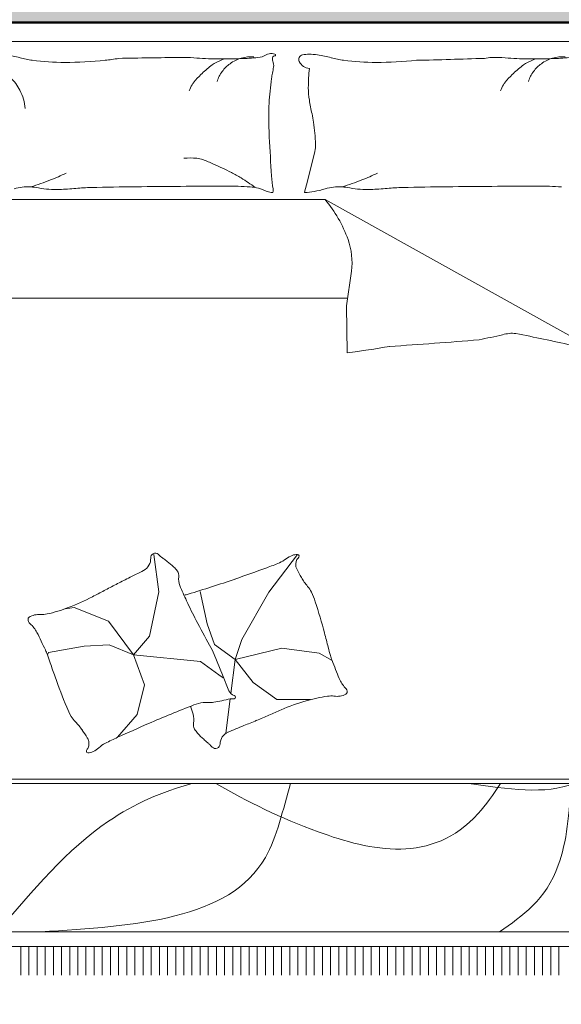
# Model space of a CAD drawing. Units: inches. Extents: x -7 to 1228, y -146 to 1091.
# Tile 11 of 88: x 105 to 153, y 401 to 487. Entities that reach past the tile are written whole.
import ezdxf

# ---------------------------------------------------------------- set-up
doc = ezdxf.new("R2010")
doc.units = ezdxf.units.IN
for name, color, linetype, lineweight in [('A-ANNO-DIMS', 2, 'Continuous', 18), ('A-FURN', 8, 'Continuous', 18), ('A-WALL', 7, 'Continuous', 50), ('A-WALL-PATT', 251, 'Continuous', 13)]:
    doc.layers.add(name, color=color, linetype=linetype, lineweight=lineweight)
doc.styles.add('DIM_FONT', font='SIMPLEX.shx', dxfattribs={"width": 0.8})
doc.styles.get("Standard").update_dxf_attribs({"font": 'arial.ttf'})
doc.dimstyles.new('ISO-25', dxfattribs={"dimtxt": 7, "dimasz": 4, "dimexe": 1.25, "dimexo": 0.625, "dimtad": 1, "dimdec": 1, "dimlunit": 3, "dimtxsty": 'Standard', "dimcen": 2.5, "dimadec": 0, "dimazin": 0, "dimtfac": 1, "dimtdec": 1, "dimtmove": 1, "dimatfit": 3, "dimfxl": 1, "dimarcsym": 0})

# ---------------------------------------------------------------- blocks, each defined once
blk = doc.blocks.new('A$C4F634EDD')
for p, q in [((0.5, 2.6295), (2.3, 2.6295)), ((0.5, 2.5771), (2.3, 2.5771)), ((1.4546, 2.1912), (1.4752, 2.2738)), ((1.4471, 2.1612), (1.4546, 2.1912)), ((1.5035, 2.141), (0.5458, 2.141)), ((1.5035, 2.141), (2.2716, 1.7136)), ((1.576, 1.9433), (1.5624, 1.8479)), ((0.5458, 1.8684), (1.5653, 1.8684)), ((1.5624, 1.8479), (1.5641, 1.7178)), ((1.031, 1.1612), (1.0448, 1.0581)), ((1.4276, 1.1611), (1.3484, 1.0571)), ((1.0448, 1.0581), (1.019, 0.936)), ((1.1784, 0.9702), (1.1586, 1.0591)), ((1.3484, 1.0571), (1.2733, 0.9268)), ((0.8108, 1.0151), (0.7868, 1.0117)), ((0.9054, 0.9773), (0.8108, 1.0151)), ((0.9743, 0.8845), (0.9054, 0.9773)), ((1.1982, 0.9129), (1.1784, 0.9702)), ((1.019, 0.936), (0.9743, 0.8845)), ((1.2733, 0.9268), (1.2555, 0.8715)), ((0.8384, 0.9085), (0.7403, 0.8913)), ((0.9072, 0.912), (0.8384, 0.9085)), ((0.9743, 0.8845), (0.9072, 0.912)), ((1.2555, 0.8715), (1.1982, 0.9129)), ((1.2555, 0.8715), (1.384, 0.9031)), ((1.384, 0.9031), (1.4868, 0.8892)), ((0.7403, 0.8913), (0.737, 0.8849)), ((0.9743, 0.8845), (1.0052, 0.802)), ((0.9743, 0.8845), (1.16, 0.8656)), ((1.1973, 0.8853), (1.2203, 0.829)), ((1.2555, 0.8715), (1.2437, 0.7773)), ((1.2555, 0.8715), (1.3049, 0.8082)), ((1.4868, 0.8892), (1.5228, 0.8692)), ((1.16, 0.8656), (1.2099, 0.8295)), ((1.2099, 0.8295), (1.222, 0.8209)), ((1.2203, 0.829), (1.2381, 0.7855)), ((1.0052, 0.802), (0.9846, 0.7194)), ((1.3049, 0.8082), (1.3701, 0.7608)), ((1.2419, 0.7626), (1.23, 0.668)), ((1.3701, 0.7608), (1.463, 0.7608)), ((0.9846, 0.7194), (0.931, 0.6569)), ((2.3, 0.5295), (0.5, 0.5295)), ((0.5458, 0.5417), (2.2516, 0.5417)), ((2.4188, 0.12), (0.3786, 0.12)), ((2.4588, 0.08), (0.3386, 0.08)), ((0.6636, 0), (0.6636, 0.08)), ((0.6861, 0), (0.6861, 0.08)), ((0.7086, 0), (0.7086, 0.08)), ((0.7311, 0), (0.7311, 0.08)), ((0.7536, 0), (0.7536, 0.08)), ((0.7761, 0), (0.7761, 0.08)), ((0.7986, 0), (0.7986, 0.08)), ((0.8211, 0), (0.8211, 0.08)), ((0.8436, 0), (0.8436, 0.08)), ((0.8661, 0), (0.8661, 0.08)), ((0.8886, 0), (0.8886, 0.08)), ((0.9111, 0), (0.9111, 0.08)), ((0.9336, 0), (0.9336, 0.08)), ((0.9561, 0), (0.9561, 0.08)), ((0.9786, 0), (0.9786, 0.08)), ((1.0011, 0), (1.0011, 0.08)), ((1.0236, 0), (1.0236, 0.08)), ((1.0461, 0), (1.0461, 0.08)), ((1.0686, 0), (1.0686, 0.08)), ((1.0911, 0), (1.0911, 0.08)), ((1.1136, 0), (1.1136, 0.08)), ((1.1361, 0), (1.1361, 0.08)), ((1.1586, 0), (1.1586, 0.08)), ((1.1811, 0), (1.1811, 0.08)), ((1.2036, 0), (1.2036, 0.08)), ((1.2261, 0), (1.2261, 0.08)), ((1.2486, 0), (1.2486, 0.08)), ((1.2711, 0), (1.2711, 0.08)), ((1.2936, 0), (1.2936, 0.08)), ((1.3161, 0), (1.3161, 0.08)), ((1.3386, 0), (1.3386, 0.08)), ((1.3611, 0), (1.3611, 0.08)), ((1.3836, 0), (1.3836, 0.08)), ((1.4061, 0), (1.4061, 0.08)), ((1.4286, 0), (1.4286, 0.08)), ((1.4511, 0), (1.4511, 0.08)), ((1.4736, 0), (1.4736, 0.08)), ((1.4961, 0), (1.4961, 0.08)), ((1.5186, 0), (1.5186, 0.08)), ((1.5411, 0), (1.5411, 0.08)), ((1.5636, 0), (1.5636, 0.08)), ((1.5861, 0), (1.5861, 0.08)), ((1.6086, 0), (1.6086, 0.08)), ((1.6311, 0), (1.6311, 0.08)), ((1.6536, 0), (1.6536, 0.08)), ((1.6761, 0), (1.6761, 0.08)), ((1.6986, 0), (1.6986, 0.08)), ((1.7211, 0), (1.7211, 0.08)), ((1.7436, 0), (1.7436, 0.08)), ((1.7661, 0), (1.7661, 0.08)), ((1.7886, 0), (1.7886, 0.08)), ((1.8111, 0), (1.8111, 0.08)), ((1.8336, 0), (1.8336, 0.08)), ((1.8561, 0), (1.8561, 0.08)), ((1.8786, 0), (1.8786, 0.08)), ((1.9011, 0), (1.9011, 0.08)), ((1.9236, 0), (1.9236, 0.08)), ((1.9461, 0), (1.9461, 0.08)), ((1.9686, 0), (1.9686, 0.08)), ((1.9911, 0), (1.9911, 0.08)), ((2.0136, 0), (2.0136, 0.08)), ((2.0361, 0), (2.0361, 0.08)), ((2.0586, 0), (2.0586, 0.08)), ((2.0811, 0), (2.0811, 0.08)), ((2.1036, 0), (2.1036, 0.08)), ((2.1261, 0), (2.1261, 0.08)), ((2.1486, 0), (2.1486, 0.08))]:
    blk.add_line(p, q)
for centre, radius, start, end in [((0.5788, 2.2388), 0.3048, 74.256, 81.5628), ((0.7272, 2.7653), 0.2422, 254.256, 262.4531), ((0.8402, 3.0514), 0.5293, 276.0867, 280.1899), ((1.1602, -8.1346), 10.6675, 90.30153, 91.21582), ((1.1169, 2.2433), 0.2897, 85.1982, 92.5386), ((1.2142, 3.4021), 0.8732, 265.1982, 269.4243), ((1.3082, 2.3102), 0.234, 110.8603, 117.2396), ((1.2204, 4.0232), 1.4943, 269.4243, 271.9079), ((1.2995, 2.4357), 0.0992, 105.9352, 126.0864), ((1.2429, 3.3501), 0.8208, 271.9079, 275.2592), ((1.2995, 2.4357), 0.0992, 85.7841, 105.9352), ((1.3132, 2.5864), 0.0539, 275.2592, 300.6513), ((1.3554, 2.5152), 0.0289, 85.6975, 120.6513), ((1.3556, 2.519), 0.0251, 68.2117, 85.6975), ((1.3739, 2.5288), 0.0156, 158.0096, 201.421), ((1.3634, 2.533), 0.00428, 78.1069, 158.0096), ((1.3647, 2.5395), 0.00232, 258.1069, 19.564), ((1.3637, 2.5391), 0.00342, 19.564, 68.2117), ((1.444, 2.5274), 0.0131, 101.2724, 206.5805), ((1.4591, 2.4516), 0.0904, 90, 101.2724), ((1.4591, 2.3808), 0.1611, 81.5628, 90), ((1.438, 2.2388), 0.3048, 74.256, 81.5628), ((1.5865, 2.7653), 0.2422, 254.256, 262.4531), ((1.4785, 15.4878), 12.9656, 271.22425, 272.05324), ((1.97, 2.3805), 0.1524, 92.5386, 100.1899), ((1.9761, 2.2433), 0.2897, 85.1982, 92.5386), ((2.0734, 3.4021), 0.8732, 265.1982, 269.4243), ((2.1674, 2.3102), 0.234, 110.8603, 117.2396), ((2.0797, 4.0232), 1.4943, 269.4243, 271.9079), ((2.1588, 2.4357), 0.0992, 105.9352, 126.0864), ((2.1021, 3.3501), 0.8208, 271.9079, 275.2592), ((2.1588, 2.4357), 0.0992, 85.7841, 105.9352), ((0.7851, 3.2019), 0.6827, 262.4531, 270), ((0.7851, 3.5682), 1.049, 270, 276.0867), ((1.4317, 2.2032), 0.3916, 128.3886, 133.8115), ((1.2362, 2.45), 0.0768, 117.2396, 128.3886), ((1.2995, 2.4357), 0.0992, 126.0864, 143.8234), ((1.1177, 2.5413), 0.246, 347.8905, 351.8665), ((1.3288, 2.5111), 0.0328, 351.8665, 21.421), ((1.4628, 2.5368), 0.0342, 206.5805, 265.5998), ((1.949, 2.4496), 0.4918, 173.7676, 180), ((1.6443, 3.2019), 0.6827, 262.4531, 270), ((1.6443, 3.5682), 1.049, 270, 276.0867), ((2.291, 2.2032), 0.3916, 128.3886, 133.8115), ((2.0954, 2.45), 0.0768, 117.2396, 128.3886), ((2.1588, 2.4357), 0.0992, 126.0864, 143.8234), ((0.5368, 2.3783), 0.1399, 27.3988, 45.0976), ((1.3165, 2.3233), 0.2252, 133.8115, 140.9651), ((1.2995, 2.4357), 0.0992, 143.8234, 161.5603), ((2.2605, 2.3525), 0.9131, 172.3191, 176.6313), ((1.5522, 2.448), 0.1983, 167.8905, 172.3191), ((2.1757, 2.3233), 0.2252, 133.8115, 140.9651), ((2.1588, 2.4357), 0.0992, 143.8234, 161.5603), ((1.3127, 2.3625), 0.2002, 151.6832, 156.9972), ((1.1799, 2.4341), 0.0493, 140.9651, 151.6832), ((1.6611, 2.4496), 0.204, 180, 189.6844), ((2.1719, 2.3625), 0.2002, 151.6832, 156.9972), ((2.0391, 2.4341), 0.0493, 140.9651, 151.6832), ((0.5368, 2.3783), 0.1399, 16.515, 27.3988), ((0.5368, 2.3783), 0.1399, 5.6311, 16.515), ((2.0266, 2.3663), 0.6787, 176.6313, 181.6331), ((2.3295, 2.5637), 0.882, 189.6844, 192.1984), ((1.1575, 2.3103), 0.3171, 8.0051, 12.1984), ((2.7128, 2.3859), 1.3652, 181.6331, 183.055), ((0.8191, 2.2627), 0.6588, 2.6649, 8.0051), ((14.9657, 3.0398), 13.6356, 183.05496, 183.50486), ((1.4096, 2.2902), 0.0677, 345.9548, 2.6649), ((1.1303, 1.9835), 0.2721, 85.9172, 93.5552), ((1.1455, 2.197), 0.058, 69.3257, 85.9172), ((0.9871, 1.7772), 0.5066, 65.6735, 69.3257), ((0.6058, 0.9338), 1.4323, 63.5015, 65.6735), ((0.473, 2.8815), 0.7387, 291.6577, 293.4844), ((0.473, 2.8815), 0.7387, 293.4844, 295.3111), ((1.1054, 1.9358), 0.3126, 57.865, 63.5015), ((1.6762, 2.2258), 0.3212, 183.5049, 189.9984), ((1.3322, 2.8815), 0.7387, 291.6577, 293.4844), ((1.3322, 2.8815), 0.7387, 293.4844, 295.3111), ((0.6807, 2.0561), 0.1197, 96.4341, 107.3864), ((0.6836, 2.0301), 0.1459, 78.4414, 96.4341), ((0.473, 2.8815), 0.7387, 287.1982, 289.428), ((0.473, 2.8815), 0.7387, 289.428, 291.6577), ((0.9136, 0.9591), 1.2165, 92.6096, 94.6176), ((1.2501, -19.8405), 22.0183, 90.37908, 91.01965), ((1.2012, -3.5404), 5.7185, 89.7135, 90.9704), ((1.224, 1.0141), 1.164, 86.426, 89.7135), ((0.8841, 1.5835), 0.7286, 54.1737, 57.865), ((1.2875, 2.0302), 0.1459, 77.131, 86.426), ((1.5399, 2.0561), 0.1197, 96.4341, 107.3864), ((1.5429, 2.0301), 0.1459, 78.4414, 96.4341), ((1.3322, 2.8815), 0.7387, 287.1982, 289.428), ((1.3322, 2.8815), 0.7387, 289.428, 291.6577), ((1.7729, 0.9591), 1.2165, 92.6096, 94.6176), ((2.1093, -19.8405), 22.0183, 90.37908, 91.01965), ((2.0605, -3.5404), 5.7185, 89.7135, 90.9704), ((2.0833, 1.0141), 1.164, 86.426, 89.7135), ((0.759, 2.3985), 0.2301, 258.4414, 272.7491), ((0.7026, 3.5718), 1.4048, 272.7491, 274.6176), ((1.3099, 2.1283), 0.0453, 62.7159, 77.131), ((1.3658, 2.2367), 0.0767, 242.7159, 253.7788), ((1.3688, 2.247), 0.0875, 253.7788, 262.8796), ((1.3581, 2.1615), 0.00132, 262.8796, 343.3022), ((1.3409, 2.1667), 0.0193, 343.3022, 9.9984), ((1.448, 2.1609), 0.000917, 165.9551, 274.0829), ((1.4288, 2.4301), 0.2708, 274.0829, 279.4841), ((1.4355, 2.3896), 0.2297, 279.4841, 287.3864), ((1.6182, 2.3985), 0.2301, 258.4414, 272.7491), ((1.5619, 3.5718), 1.4048, 272.7491, 274.6176), ((1.2147, 1.9017), 0.3751, 20.1488, 39.6445), ((1.3977, 1.9688), 0.1801, 351.8644, 20.1488), ((1.4194, 4.2174), 2.5158, 281.6741, 283.1904), ((2.0378, 1.5789), 0.1942, 97.7304, 103.1904), ((2.0195, 1.7137), 0.0581, 79.2724, 97.7304), ((1.2737, -2.2227), 4.0646, 77.0745, 79.2724), ((0.6102, 18.0525), 16.3521, 273.75703, 274.62393), ((1.0582, 5.4638), 3.7801, 277.692, 279.495), ((0.9863, 1.1494), 0.0359, 297.2902, 3.2455), ((1.0348, 1.1521), 0.0127, 51.1864, 183.2455), ((0.9991, 1.1077), 0.0697, 45.8726, 51.1864), ((1.0791, 1.1902), 0.0452, 225.8726, 232.4713), ((1.2846, 1.4577), 0.3825, 232.4713, 233.7837), ((0.6683, 0.6162), 0.6605, 52.7849, 53.7837), ((0.9362, 0.9689), 0.2176, 46.4776, 52.7849), ((1.3469, 1.2115), 0.0792, 292.7069, 308.5854), ((1.4338, 1.1026), 0.0601, 110.3452, 128.5854), ((1.4251, 1.1259), 0.0352, 86.0516, 110.3452), ((1.4996, 1.1284), 0.0771, 169.5926, 177.2714), ((1.4376, 1.1398), 0.0142, 126.5792, 169.5926), ((1.4273, 1.1567), 0.00443, 13.2808, 86.0516), ((1.4254, 1.1562), 0.0063, 306.5792, 13.2808), ((-0.4173, 3.8699), 3.0972, 296.4147, 297.2902), ((1.0327, 1.0706), 0.0774, 35.8936, 46.4776), ((1.0771, 1.1027), 0.0226, 351.9508, 35.8936), ((-0.4107, 5.9078), 5.0942, 289.0836, 290.1287), ((1.0543, 1.9106), 0.8371, 290.1287, 292.7069), ((1.4378, 1.1314), 0.0153, 177.2714, 194.5709), ((1.4611, 1.1374), 0.0393, 194.5709, 206.8179), ((1.7401, 1.2785), 0.352, 206.8179, 210.9056), ((1.8575, -0.7096), 2.0162, 116.4147, 117.4999), ((1.1449, 1.0931), 0.0458, 171.9508, 202.4162), ((0.2266, 4.0657), 3.145, 286.6085, 289.0836), ((1.6045, 1.1973), 0.194, 210.9056, 219.7005), ((-1.8336, 6.2238), 5.8383, 297.49208, 297.84822), ((3.744, -4.3336), 6.1019, 117.49986, 117.84822), ((2.032, 1.4591), 1.0054, 202.4162, 205.0529), ((1.3929, 1.0217), 0.081, 26.0735, 39.7005), ((0.5736, 1.5979), 0.6236, 290.7486, 297.4921), ((1.0922, 1.1636), 0.1166, 280.7366, 286.6085), ((2.6493, 1.7476), 1.6868, 205.0529, 207.0884), ((1.2892, 0.9709), 0.1965, 17.8396, 26.0735), ((0.6422, 1.4168), 0.43, 282.6252, 290.7486), ((-0.4304, 0.4175), 2.003, 15.2625, 17.8396), ((0.6894, 0.9832), 0.0058, 121.6917, 179.0386), ((0.7004, 0.983), 0.0168, 179.0386, 229.4914), ((0.7131, 0.9448), 0.0509, 103.0402, 121.6917), ((0.7152, 0.9361), 0.0599, 86.6119, 103.0402), ((0.7224, 1.0587), 0.063, 266.6119, 282.6252), ((2.541, 1.6922), 1.5652, 207.0884, 209.936), ((0.6405, 0.9128), 0.0755, 26.3332, 49.4914), ((-1.6775, -0.2344), 2.6619, 25.1732, 26.3332), ((-0.0881, 0.5109), 1.6481, 13.841, 15.2625), ((0.5689, 0.8213), 0.1798, 20.7081, 25.1732), ((0.9989, 0.8042), 0.2143, 22.2355, 29.936), ((2.0418, 1.0357), 0.5454, 193.841, 196.3122), ((0.2268, 0.692), 0.5454, 18.2369, 20.7081), ((1.6908, 0.933), 0.1798, 196.3122, 200.7773), ((2.3102, 1.3785), 1.6481, 198.2369, 199.6584), ((4.0115, 1.8135), 2.6619, 200.7773, 201.9373), ((2.6444, 1.4979), 2.003, 199.6584, 202.2355), ((1.6124, 0.8472), 0.0755, 201.9373, 225.0955), ((1.5473, 0.7819), 0.0168, 354.6428, 45.0955), ((1.2689, 0.569), 0.1955, 97.9822, 104.8807), ((1.2594, 0.7942), 0.0231, 202.2355, 252.8133), ((1.2465, 0.729), 0.034, 85.7407, 97.9822), ((1.2497, 0.772), 0.0092, 265.7407, 289.3799), ((1.2512, 0.7678), 0.00467, 289.3799, 72.8133), ((1.5721, 0.3449), 0.43, 98.2293, 106.3527), ((1.5195, 0.708), 0.063, 82.216, 98.2293), ((1.5362, 0.8298), 0.0599, 262.216, 278.6443), ((1.5375, 0.8209), 0.0509, 278.6443, 297.2959), ((1.5582, 0.7808), 0.0058, 297.2959, 354.6428), ((0.9722, 0.8143), 0.1965, 202.2355, 210.4694), ((2.2689, -2.1899), 3.145, 111.0043, 113.4795), ((0.1831, 0.4093), 1.0054, 18.0203, 19.3448), ((1.1834, 0.6373), 0.1166, 98.1216, 111.0043), ((1.1763, 0.687), 0.0663, 85.4882, 98.1216), ((1.1871, 0.8241), 0.0712, 265.4882, 277.6784), ((1.1727, 0.9313), 0.1794, 277.6784, 284.8807), ((1.6266, 0.159), 0.6236, 106.3527, 113.0962), ((0.8727, 0.7557), 0.081, 210.4694, 224.0964), ((1.0957, 0.7061), 0.0458, 347.5549, 18.0203), ((-1.0798, 6.3161), 6.1019, 293.10398, 293.45234), ((3.6722, -4.6377), 5.8383, 113.0962, 113.45234), ((0.6752, 0.5644), 0.194, 35.3015, 44.0964), ((3.0455, -3.9778), 5.0942, 113.4795, 114.5246), ((1.1625, 0.6914), 0.0226, 167.5549, 211.4977), ((1.2092, 0.72), 0.0774, 211.4977, 222.0817), ((2.4404, -2.1823), 3.0972, 112.0188, 112.8944), ((0.5234, 2.5582), 2.0162, 292.0188, 293.104), ((0.5462, 0.4731), 0.352, 31.2138, 35.3015), ((0.8136, 0.6351), 0.0393, 18.9668, 31.2138), ((1.2784, -0.1047), 0.8371, 114.5246, 117.1028), ((1.3133, 0.814), 0.2176, 222.0817, 228.389), ((1.2495, 0.6379), 0.0359, 112.8944, 178.8496), ((0.8372, 0.6345), 0.0142, 310.9751, 353.9885), ((0.8364, 0.6429), 0.0153, 1.6673, 18.9668), ((0.7746, 0.6411), 0.0771, 353.9885, 1.6673), ((0.8382, 0.6719), 0.0601, 294.7411, 312.9813), ((0.9332, 0.57), 0.0792, 117.1028, 132.9813), ((1.6074, 1.1451), 0.6605, 228.389, 229.3878), ((0.9284, 0.3533), 0.3825, 48.0754, 49.3878), ((1.1538, 0.6043), 0.0452, 41.4767, 48.0754), ((1.2399, 0.6804), 0.0697, 221.4767, 226.7905), ((1.2009, 0.6389), 0.0127, 226.7905, 358.8496), ((0.8506, 0.6191), 0.0063, 130.9751, 197.6767), ((0.8488, 0.6185), 0.00443, 197.6767, 270.4475), ((0.8486, 0.6493), 0.0352, 270.4475, 294.7411)]:
    blk.add_arc(centre, radius, start, end)
for points, knots in [([(0.5992, 0.12), (0.6957, 0.2341), (0.8523, 0.4189), (1.0536, 0.5069), (1.136, 0.5295)], [0, 0, 0, 0, 432.822832, 701.445452, 701.445452, 701.445452, 701.445452]), ([(0.7187, 0.12), (0.9791, 0.1362), (1.326, 0.1577), (1.3868, 0.4574), (1.408, 0.5295)], [0, 0, 0, 0, 653.160442, 870.050857, 870.050857, 870.050857, 870.050857]), ([(1.2016, 0.5295), (1.2892, 0.479), (1.5144, 0.3684), (1.8265, 0.2994), (1.9681, 0.4992), (1.9875, 0.5295)], [936.534237, 936.534237, 936.534237, 936.534237, 1243.285375, 1683.261222, 1758.254386, 1758.254386, 1758.254386, 1758.254386]), ([(2.1796, 0.5295), (2.1798, 0.4519), (2.1548, 0.2369), (2.0487, 0.164), (1.9846, 0.12)], [2202.034493, 2202.034493, 2202.034493, 2202.034493, 2357.807635, 2594.446174, 2594.446174, 2594.446174, 2594.446174])]:
    blk.add_open_spline(points, degree=3, knots=knots)
blk.add_open_spline([(1.9003, 0.5295), (2.0065, 0.514), (2.1132, 0.4978), (2.1894, 0.5295)], degree=3)
at = {"style": 'DIM_FONT', "width": 0.8, "flags": 9}
for tag, p in [('YSIZE', (0.5, 2.6295)), ('XSIZE', (0.5, 2.6295)), ('XSIZE', (2.2985, 2.6295)), ('YSIZE', (2.2985, 2.6295))]:
    blk.add_attdef(tag, p, '', height=0.0005, dxfattribs=at)
blk = doc.blocks.new('*D24')
at = {"layer": 'A-ANNO-DIMS', "color": 0, "lineweight": -2, "transparency": 16777216}
for p, q in [((84.435, 402.798), (84.435, 388.824)), ((173.431, 402.798), (173.431, 388.824)), ((88.435, 390.074), (169.431, 390.074))]:
    blk.add_line(p, q, dxfattribs=at)
at = {"layer": 'A-ANNO-DIMS', "color": 0, "transparency": 16777216}
for points in [[(88.435, 390.741), (88.435, 389.407), (84.435, 390.074)], [(169.431, 390.741), (169.431, 389.407), (173.431, 390.074)]]:
    blk.add_solid(points, dxfattribs=at)
at = {"layer": 'Defpoints', "color": 0, "transparency": 16777216}
for p in [(84.435, 403.423), (173.431, 403.423), (173.431, 390.074)]:
    blk.add_point(p, dxfattribs=at)
at = {"layer": 'A-ANNO-DIMS', "color": 0, "transparency": 16777216, "insert": (128.933, 394.259), "char_height": 7, "attachment_point": 5}
blk.add_mtext('BED 7\'-5" TYP.', dxfattribs=at)

msp = doc.modelspace()

# ---------------------------------------------------------------- hatches: boundary and pattern name
at = {"layer": 'A-WALL-PATT'}
h = msp.add_hatch(color=256, dxfattribs=at)
h.dxf.hatch_style = 1
h.paths.add_polyline_path([(69, 568), (60, 568), (60, 493), (63.289, 493), (69, 493)])
h.paths.add_polyline_path([(69, 662.405), (60, 662.405), (60, 586), (69, 586)], flags=17)
h.paths.add_polyline_path([(69, 723), (184, 723), (184, 734), (179, 734), (179, 728), (69, 728), (69, 741.623), (60, 741.623), (60, 698.405), (69, 698.405)], flags=17)
h.paths.add_polyline_path([(69, 782), (231, 782), (231, 728), (231, 723), (231, 586), (236, 586), (236, 787), (69, 787), (69, 800.126), (60, 800.126), (60, 765.623), (69, 765.623)])
h.paths.add_polyline_path([(184, 842), (189, 842), (189, 848), (173, 848), (173, 842), (179, 842), (179, 787), (184, 787)])
h.paths.add_polyline_path([(118.22, 69), (69, 69), (69, 60), (118.22, 60)])
h.paths.add_polyline_path([(227, 69), (154.22, 69), (154.22, 60), (227, 60)])
h.paths.add_polyline_path([(236, 60), (232.711, 60), (227, 60), (227, 36), (236, 36)])
h.paths.add_polyline_path([(389, 60), (380, 60), (380, 36), (389, 36)])
h.paths.add_polyline_path([(384, 181), (380, 181), (380, 115), (380, 78), (384, 78)])
h.paths.add_polyline_path([(380, 115), (334.547, 115), (334.547, 109), (380, 109)])
h.paths.add_polyline_path([(274.547, 115), (236, 115), (236, 201), (232.711, 201), (231, 201), (231, 78), (236, 78), (236, 109), (274.547, 109)])
h.paths.add_polyline_path([(69, 123), (60, 123), (60, 78), (69, 78)])
h.paths.add_polyline_path([(69, 201), (60, 201), (60, 159), (69, 159)])
h.paths.add_polyline_path([(143, 219), (69, 219), (69, 213), (143, 213)], flags=17)
h.paths.add_polyline_path([(189, 219), (184, 219), (184, 274), (231, 274), (231, 219), (236, 219), (236, 279), (184, 279), (184, 297), (179, 297), (179, 279), (69, 279), (69, 290.912), (60, 290.912), (60, 262.179), (69, 262.179), (69, 274), (179, 274), (179, 219), (173, 219), (173, 213), (189, 213)])
h.paths.add_polyline_path([(69, 238.179), (60, 238.179), (60, 219), (69, 219)], flags=17)
h.paths.add_polyline_path([(69, 333), (60, 333), (60, 314.912), (69, 314.912), (69, 316.965)])
h.paths.add_polyline_path([(190, 338), (184, 338), (69, 338), (69, 333), (179, 333), (179, 327), (184, 327), (184, 333.021), (190, 333.046)])
h.paths.add_polyline_path([(69, 386.806), (60, 386.806), (60, 351), (69, 351)])
h.paths.add_polyline_path([(69, 475), (60, 475), (60, 422.806), (69, 422.806)])
h.paths.add_polyline_path([(236, 475), (231, 475), (231, 351.238), (236, 351.238)])
h.paths.add_polyline_path([(384, 475), (380, 475), (380, 362), (384, 362)])
h.paths.add_polyline_path([(547, 307), (439, 307), (439, 356), (445, 356), (445, 362), (433, 362), (433, 307), (380, 307), (380, 244), (380, 241), (384, 241), (384, 301), (433, 301), (433, 277), (439, 277), (439, 301), (547, 301)])
h.paths.add_polyline_path([(547, 241), (439, 241), (439, 247), (433, 247), (433, 235), (547, 235)])
h.paths.add_polyline_path([(450, 69), (440.286, 69), (424.889, 69), (389, 69), (389, 60), (450, 60)])
h.paths.add_polyline_path([(547, 69), (486, 69), (486, 60), (547, 60)])
h.paths.add_polyline_path([(556, 148.268), (547, 148.268), (547, 78), (556, 78)])
h.paths.add_polyline_path([(556, 223), (547, 223), (547, 195), (547, 184.268), (556, 184.268)])
h.paths.add_polyline_path([(556, 311.192), (547, 311.192), (547, 273.075), (556, 273.075)])
h.paths.add_polyline_path([(556, 344), (552.711, 344), (547, 344), (547, 335.192), (556, 335.192)])
h.paths.add_polyline_path([(556, 249.075), (547, 249.075), (547, 241), (556, 241)])
h.paths.add_polyline_path([(547, 362), (475, 362), (475, 356), (547, 356)], flags=0)
h.paths.add_polyline_path([(556, 399.621), (547, 399.621), (547, 362), (556, 362)])
h.paths.add_polyline_path([(556, 475), (547, 475), (547, 435.621), (556, 435.621)])
h.paths.add_polyline_path([(547, 493), (389, 493), (389, 487), (547, 487)])
h.paths.add_polyline_path([(380, 493), (278, 493), (278, 487), (380, 487)])
h.paths.add_polyline_path([(227, 493), (69, 493), (69, 487), (227, 487)])
h.paths.add_polyline_path([(643, 122.445), (634, 122.445), (634, 78), (643, 78)])
h.paths.add_polyline_path([(702.5, 69), (692.786, 69), (677.389, 69), (643, 69), (643, 60), (702.5, 60)])
h.paths.add_polyline_path([(798, 69), (738.5, 69), (738.5, 60), (798, 60)])
h.paths.add_polyline_path([(807, 60), (803.711, 60), (798, 60), (798, 36), (807, 36)])
h.paths.add_polyline_path([(807, 109), (846.751, 109), (846.751, 115), (807, 115), (807, 159), (802, 159), (802, 78), (807, 78)])
h.paths.add_polyline_path([(807, 201), (802, 201), (802, 195), (807, 195)])
h.paths.add_polyline_path([(643, 201), (634, 201), (634, 158.445), (643, 158.445)])
h.paths.add_polyline_path([(756, 225), (751, 225), (751, 219), (643, 219), (643, 213), (756, 213)])
h.paths.add_polyline_path([(643, 240.848), (634, 240.848), (634, 219), (643, 219)])
h.paths.add_polyline_path([(643, 274), (643, 288.629), (634, 288.629), (634, 264.848), (643, 264.848)])
h.paths.add_polyline_path([(802, 279), (756, 279), (756, 297), (751, 297), (751, 279), (643, 279), (643, 274), (751, 274), (751, 255), (756, 255), (756, 274), (802, 274)])
h.paths.add_polyline_path([(807, 333), (803.711, 333), (802, 333), (802, 279), (802, 274), (802, 219), (807, 219)])
h.paths.add_polyline_path([(956, 182), (951, 182), (951, 115), (906.751, 115), (906.751, 109), (951, 109), (951, 78), (956, 78)])
h.paths.add_polyline_path([(960, 60), (951, 60), (951, 36), (960, 36)])
h.paths.add_polyline_path([(1021, 69), (1005.781, 69), (960, 69), (960, 60), (1021, 60)])
h.paths.add_polyline_path([(956, 224), (951, 224), (951, 218), (956, 218)])
h.paths.add_polyline_path([(956, 302), (1004, 302), (1004, 278), (1010, 278), (1010, 302), (1118, 302), (1118, 290.809), (1127, 290.809), (1127, 326.968), (1118, 326.968), (1118, 320.966), (1118, 307), (1010, 307), (1010, 356), (1016, 356), (1016, 362), (1004, 362), (1004, 307), (951, 307), (951, 244), (951, 242), (954.289, 242), (956, 242)])
h.paths.add_polyline_path([(643, 333), (634, 333), (634, 312.629), (643, 312.629), (643, 316.965)])
h.paths.add_polyline_path([(756, 338), (643, 338), (643, 333), (751, 333), (751, 327), (756, 327)])
h.paths.add_polyline_path([(643, 388), (634, 388), (634, 351), (643, 351)])
h.paths.add_polyline_path([(807, 357), (802, 357), (802, 351), (807, 351)])
h.paths.add_polyline_path([(807, 475), (802, 475), (802, 393), (807, 393)])
h.paths.add_polyline_path([(643, 475), (634, 475), (634, 424), (643, 424)])
h.paths.add_polyline_path([(798, 493), (643, 493), (643, 487), (798, 487)])
h.paths.add_polyline_path([(634, 493), (556, 493), (556, 487), (634, 487)])
h.paths.add_polyline_path([(813, 493), (807, 493), (807, 487), (813, 487)])
h.paths.add_polyline_path([(951, 493), (849, 493), (849, 487), (951, 487)])
h.paths.add_polyline_path([(956, 484), (951, 484), (951, 374), (956, 374)])
h.paths.add_polyline_path([(1109, 493), (969, 493), (969, 487), (1109, 487)])
h.paths.add_polyline_path([(1127, 484), (1118, 484), (1118, 450.641), (1127, 450.641)])
h.paths.add_polyline_path([(1127, 414.641), (1118, 414.641), (1118, 365), (1127, 365)])
h.paths.add_polyline_path([(1109, 362), (1046, 362), (1046, 356), (1109, 356)], flags=17)
h.paths.add_polyline_path([(1127, 356), (1123.454, 356), (1118, 356), (1118, 350.968), (1127, 350.968)], flags=0)
h.paths.add_polyline_path([(1127, 266.809), (1118, 266.809), (1118, 262.361), (1118, 242), (1127, 242)], flags=17)
h.paths.add_polyline_path([(1118, 242), (1010, 242), (1010, 248), (1004, 248), (1004, 237), (1118, 237)])
h.paths.add_polyline_path([(1127, 224), (1118, 224), (1118, 170), (1127, 170)])
h.paths.add_polyline_path([(1127, 134), (1118, 134), (1118, 78), (1127, 78)])
h.paths.add_polyline_path([(1118, 69), (1057, 69), (1057, 60), (1118, 60)])
h.paths.add_polyline_path([(227, 571.546), (227, 574), (69, 574), (69, 568), (227, 568)])
h.paths.add_polyline_path([(380, 571.546), (380, 574), (278, 574), (278, 568), (380, 568)])
h.paths.add_polyline_path([(242, 574), (236, 574), (236, 568), (242, 568)])
h.paths.add_polyline_path([(547, 571.546), (547, 574), (389, 574), (389, 568), (547, 568)])
h.paths.add_polyline_path([(384, 733), (380, 733), (380, 586), (384, 586)])
h.paths.add_polyline_path([(556, 646), (634, 646), (634, 655), (547, 655), (547, 586), (556, 586)])
h.paths.add_polyline_path([(634, 574), (556, 574), (556, 568), (634, 568)])
h.paths.add_polyline_path([(643, 655), (634, 655), (634, 586), (643, 586)])
h.paths.add_polyline_path([(798, 574), (643, 574), (643, 568), (798, 568)])
h.paths.add_polyline_path([(643, 663.854), (634, 663.854), (634, 655), (643, 655)])
h.paths.add_polyline_path([(556, 676.967), (547, 676.967), (547, 655), (556, 655)])
h.paths.add_polyline_path([(556, 733), (547, 733), (547, 712.967), (556, 712.967)])
h.paths.add_polyline_path([(643, 710), (634, 710), (634, 699.854), (643, 699.854)])
h.paths.add_polyline_path([(807, 668), (802, 668), (802, 586), (807, 586)])
h.paths.add_polyline_path([(951, 574), (849, 574), (849, 568), (951, 568)])
h.paths.add_polyline_path([(956, 691), (951, 691), (951, 577), (956, 577)])
h.paths.add_polyline_path([(1109, 574), (969, 574), (969, 568), (1109, 568)])
h.paths.add_polyline_path([(1127, 643.403), (1118, 643.403), (1118, 577), (1127, 577)])
h.paths.add_polyline_path([(1127, 568), (1123.454, 568), (1118, 568), (1118, 493), (1127, 493)])
h.paths.add_polyline_path([(1127, 733), (1118, 733), (1118, 679.403), (1127, 679.403)])
h.paths.add_polyline_path([(1127, 777.348), (1118, 777.348), (1118, 770.035), (1118, 751), (1127, 751)], flags=17)
h.paths.add_polyline_path([(1118, 751), (1010, 751), (1010, 757), (1004, 757), (1004, 745), (1118, 745)])
h.paths.add_polyline_path([(956, 811), (1004, 811), (1004, 787), (1010, 787), (1010, 811), (1017.874, 811), (1017.874, 811.627, -0.414214), (1018.247, 812), (1031.978, 812, -0.414214), (1032.351, 811.627), (1032.351, 811), (1118, 811), (1118, 801.348), (1127, 801.348), (1127, 834.685), (1118, 834.685), (1118, 830.238), (1118, 817), (1010, 817), (1010, 866), (1016, 866), (1016, 872), (1004, 872), (1004, 817), (956, 817), (956, 866), (951, 866), (951, 751), (954.289, 751), (956, 751)])
h.paths.add_polyline_path([(1118, 872), (1046, 872), (1046, 866), (1118, 866)], flags=17)
h.paths.add_polyline_path([(1127, 924.711), (1118, 924.711), (1118, 884), (1127, 884)])
h.paths.add_polyline_path([(1127, 866), (1123.711, 866), (1118, 866), (1118, 858.685), (1127, 858.685)], flags=17)
h.paths.add_polyline_path([(956, 983), (951, 983), (951, 952), (807, 952), (807, 983), (802, 983), (802, 902), (807, 902), (807, 946), (951, 946), (951, 884), (956, 884)])
h.paths.add_polyline_path([(807, 842), (802, 842), (802, 787), (756, 787), (756, 806), (751, 806), (751, 787), (643, 787), (643, 782), (751, 782), (751, 764), (756, 764), (756, 782), (802, 782), (802, 728), (807, 728)])
h.paths.add_polyline_path([(756, 848), (643, 848), (643, 842), (751, 842), (751, 836), (756, 836)])
h.paths.add_polyline_path([(756, 734), (751, 734), (751, 728), (643, 728), (643, 723), (756, 723)])
h.paths.add_polyline_path([(643, 749.791), (634, 749.791), (634, 728), (637.289, 728), (643, 728)])
h.paths.add_polyline_path([(643, 805.405), (634, 805.405), (634, 773.791), (643, 773.791)])
h.paths.add_polyline_path([(643, 896.663), (634, 896.663), (634, 860), (637.289, 860), (643, 860)])
h.paths.add_polyline_path([(643, 842), (634, 842), (634, 829.405), (643, 829.405)])
h.paths.add_polyline_path([(643, 983), (634, 983), (634, 932.663), (643, 932.663)])
h.paths.add_polyline_path([(1127, 983), (1118, 983), (1118, 960.711), (1127, 960.711)])
h.paths.add_polyline_path([(1118, 1001), (1077.525, 1001), (1077.525, 992), (1118, 992)])
h.paths.add_polyline_path([(1041.525, 1001), (960, 1001), (960, 992), (1041.525, 992)])
h.paths.add_polyline_path([(960, 1025), (951, 1025), (951, 1001), (954.289, 1001), (960, 1001)])
h.paths.add_polyline_path([(807, 1025), (798, 1025), (798, 1001), (807, 1001)])
h.paths.add_polyline_path([(798, 1001), (738.5, 1001), (738.5, 992), (798, 992)])
h.paths.add_polyline_path([(702.5, 1001), (643, 1001), (643, 992), (702.5, 992)])
h.paths.add_polyline_path([(547, 1001), (499.113, 1001), (499.113, 992), (547, 992)])
h.paths.add_polyline_path([(463.113, 1001), (389, 1001), (389, 992), (463.113, 992)])
h.paths.add_polyline_path([(389, 1025), (380, 1025), (380, 1022), (380, 1001), (383.289, 1001), (389, 1001)])
h.paths.add_polyline_path([(236, 1025), (227, 1025), (227, 1001), (236, 1001)])
h.paths.add_polyline_path([(236, 983), (231, 983), (231, 860), (236, 860)])
h.paths.add_polyline_path([(274.547, 952), (236, 952), (236, 946), (274.547, 946)])
h.paths.add_polyline_path([(380, 952), (334.547, 952), (334.547, 946), (380, 946)])
h.paths.add_polyline_path([(384, 983), (380, 983), (380, 884), (383.289, 884), (384, 884)])
h.paths.add_polyline_path([(227, 1001), (155.012, 1001), (155.012, 992), (162.875, 992), (227, 992)])
h.paths.add_polyline_path([(119.012, 1001), (69, 1001), (69, 992), (119.012, 992)])
h.paths.add_polyline_path([(69, 983), (60, 983), (60, 922.987), (69, 922.987)])
h.paths.add_polyline_path([(69, 886.987), (60, 886.987), (60, 860), (63.289, 860), (69, 860)])
h.paths.add_polyline_path([(143, 848), (69, 848), (69, 842), (143, 842)])

# ---------------------------------------------------------------- linework, layer by layer
at = {"layer": 'A-WALL'}
msp.add_line((231, 487), (69, 487), dxfattribs=at)

# ---------------------------------------------------------------- block references
at = {"layer": 'A-FURN', "xscale": 31.78426361944092, "yscale": 31.78426361944092, "zscale": 31.78426361944092}
msp.add_blockref('A$C4F634EDD', (84.435, 403.423), dxfattribs=at)

# ---------------------------------------------------------------- dimensions: what is measured, and where the dimension line sits
at = {"layer": 'A-ANNO-DIMS'}
dim = msp.add_linear_dim(base=(173.431, 390.074), p1=(84.435, 403.423), p2=(173.431, 403.423), text='BED <> TYP.', dimstyle='ISO-25', override={"dimdec": 1, "dimlfac": 1, "dimrnd": 0, "dimzin": 1, "dimdsep": 46, "dimlunit": 4, "dimfrac": 2}, dxfattribs=at)
dim.commit()
dim.dimension.update_dxf_attribs({"geometry": '*D24', "text_midpoint": (128.933, 394.259)})

doc.saveas('drawing.dxf')
